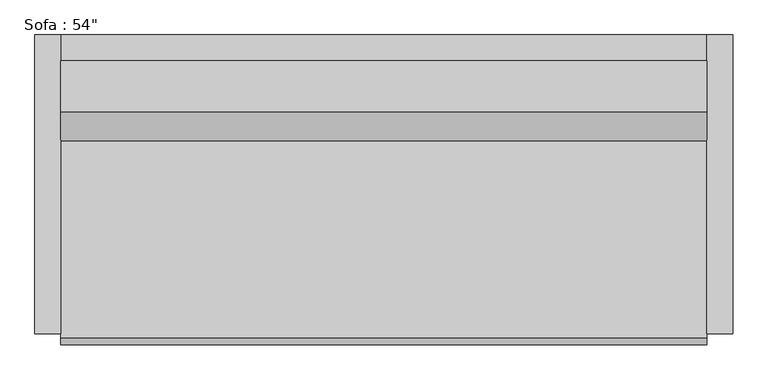
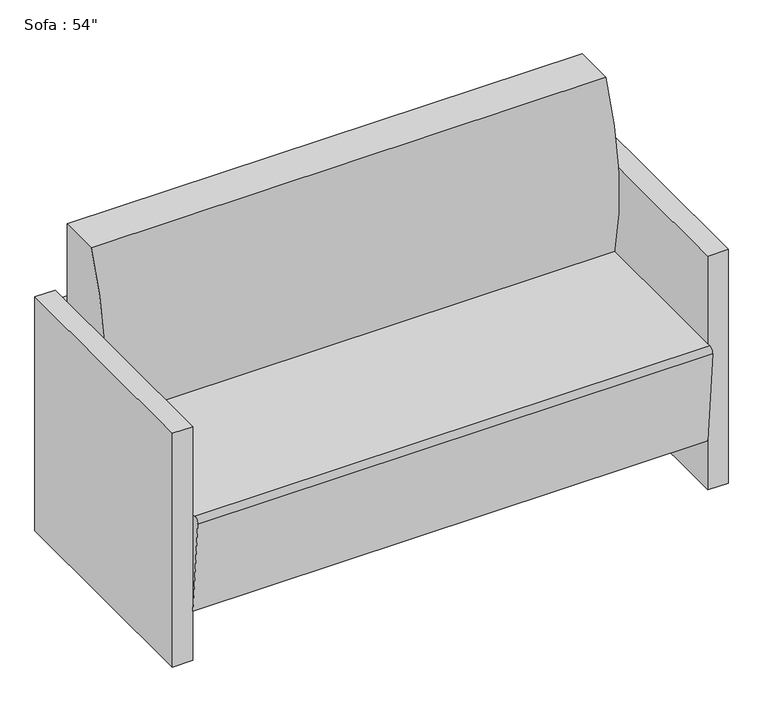
"""IFC4 building model written with IfcOpenShell, lengths in millimetres: furniture geometry."""

from ifc_helpers import new_model, si_unit, point, frame, frame_2d, origin, origin_with_axes, place, context, project, spatial, polyline, circle_curve, trimmed, segment, composite_curve, outline, extrude, source, transform, mapped, element, save


def furniture_de36dbc2(model_context):
    return source(origin(), model_context, "Body", "SweptSolid", [
        extrude(outline(polyline([(-564.6295082, 425.5540984), (-564.6295082, 476.3540984), (705.3704918, 476.3540984), (705.3704918, 425.5540984), (-564.6295082, 425.5540984)])), frame((0.0, 0.0, 457.2), z_axis=(0.0, 0.0, 1.0), x_axis=(1.0, 0.0, 0.0)), (0.0, 0.0, 1.0), 127.0),
        extrude(outline(polyline([(-564.6295082, 425.5540984), (-564.6295082, 476.3540984), (705.3704918, 476.3540984), (705.3704918, 425.5540984), (-564.6295082, 425.5540984)])), frame((0.0, 0.0, 266.7), z_axis=(0.0, 0.0, 1.0), x_axis=(1.0, 0.0, 0.0)), (0.0, 0.0, 1.0), 127.0),
        extrude(outline(polyline([(-564.6295082, 425.5540984), (-564.6295082, 476.3540984), (705.3704918, 476.3540984), (705.3704918, 425.5540984), (-564.6295082, 425.5540984)])), frame((0.0, 0.0, 76.2), z_axis=(0.0, 0.0, 1.0), x_axis=(1.0, 0.0, 0.0)), (0.0, 0.0, 1.0), 127.0),
        extrude(outline(composite_curve([segment(trimmed(circle_curve(frame_2d((926.517198, 542.5300036)), 660.4), [point((286.1764935, 381.0))], [point((323.9540984, 812.8))], False, "CARTESIAN"), True, "CONTINUOUS"), segment(polyline([(323.9540984, 812.8), (425.5540984, 812.8), (425.5540984, 127.9665467), (-111.108343, 127.9665467), (-132.0379563, 367.1931221)]), True, "CONTINUOUS"), segment(trimmed(circle_curve(frame_2d((-119.3862837, 368.3)), 12.7), [point((-132.0379563, 367.1931221))], [point((-119.3862837, 381.0))], False, "CARTESIAN"), True, "CONTINUOUS"), segment(polyline([(-119.3862837, 381.0), (286.1764935, 381.0)]), True, "CONTINUOUS")], self_intersect=False)), frame((-564.6295082, 0.0, 0.0), z_axis=(1.0, 0.0, 0.0), x_axis=(0.0, 1.0, 0.0)), (0.0, 0.0, 1.0), 1270.0),
        extrude(outline(polyline([(-615.4295082, 476.3540984), (-564.6295082, 476.3540984), (-564.6295082, -111.108343), (-615.4295082, -111.108343), (-615.4295082, 476.3540984)])), origin_with_axes(), (0.0, 0.0, 1.0), 609.6),
        extrude(outline(polyline([(756.1704918, 476.3540984), (756.1704918, -111.108343), (705.3704918, -111.108343), (705.3704918, 476.3540984), (756.1704918, 476.3540984)])), origin_with_axes(), (0.0, 0.0, 1.0), 609.6),
    ])


if __name__ == "__main__":
    model = new_model("IFC4")
    model_context = context("Model", 3, world=origin())
    ifc_project = project(units=[si_unit("LENGTHUNIT", "METRE", prefix="MILLI")], contexts=[model_context])
    site = spatial("IfcSite", under=ifc_project)
    building = spatial("IfcBuilding", under=site)
    placement = place(None, origin())
    furniture_shape = furniture_de36dbc2(model_context)
    element("IfcFurniture", 1, ObjectType="Sofa : 54\"", at=placement, inside=building, context=model_context, shape_type="MappedRepresentation", body=[
        mapped(furniture_shape, transform((0.0, 0.0, 0.0), x_axis=(1.0, 0.0, 0.0), y_axis=(0.0, 1.0, 0.0), z_axis=(0.0, 0.0, 1.0))),
    ])
    save(model, "model.ifc")

# Revit data of these elements
# Type "Sofa : 54\""
#   Assembly Code = "E2020200"
#   Width = 4' - 6"
#   Seat Material = none
#   Frame Material = none
#   Default Elevation = 0
# Element 1 (IfcFurniture, "Sofa : 54\"")
#   Materials on its faces: "Cherry"
# Materials
#   "Cherry": class "Wood", colour RGB 226 177 128, transparency 0, Description = "Prunus Serotina", Cost = 0
